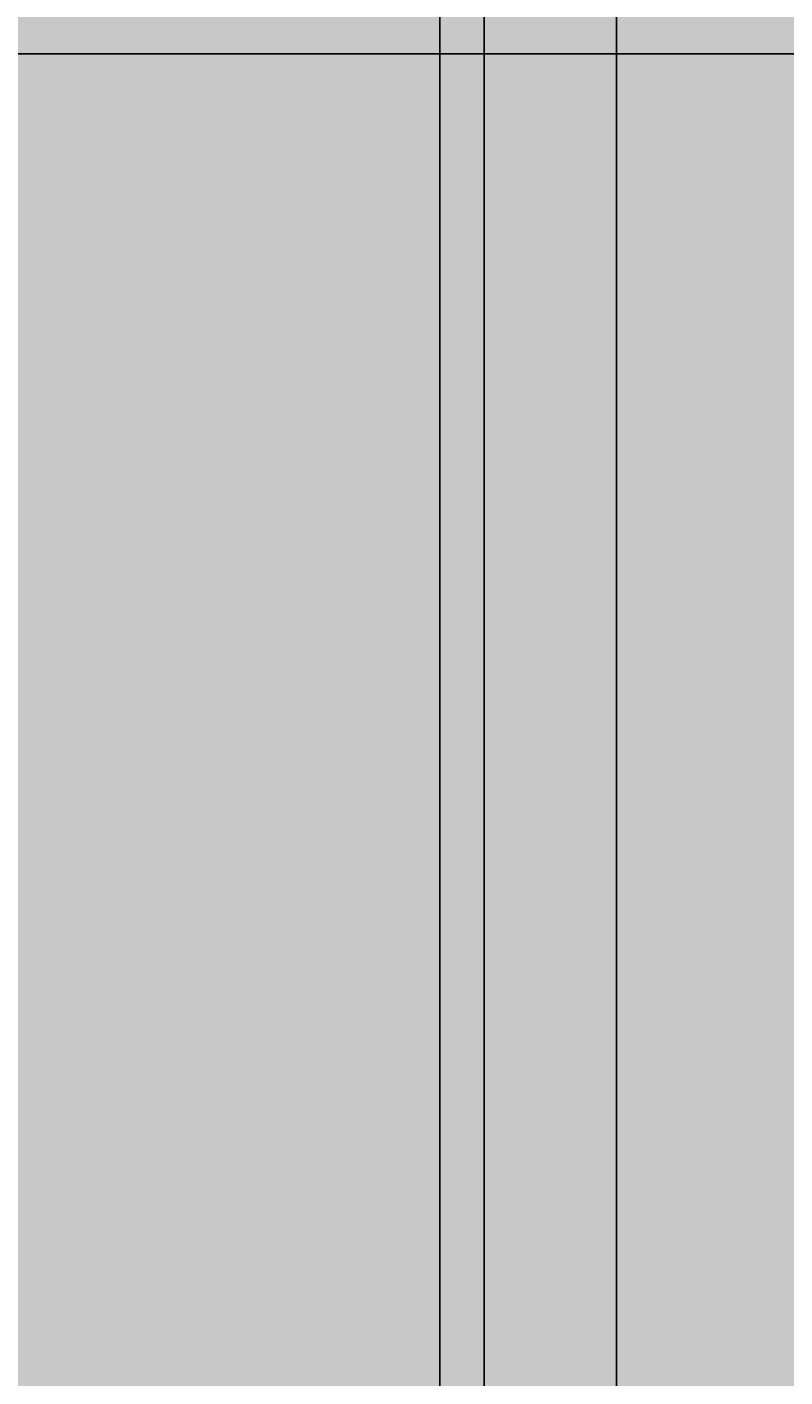
# Model space of a CAD drawing. Units: feet. Extents: x 2695 to 2912, y 795 to 1139.
# Tile 25 of 83: x 2825 to 2842, y 845 to 875. Entities that reach past the tile are written whole.
import ezdxf

# ---------------------------------------------------------------- set-up
doc = ezdxf.new("R2010")
doc.units = ezdxf.units.FT
for name, color, linetype, lineweight in [('A-ANNO-DIMS', 2, 'Continuous', 18), ('A-DOOR', 3, 'Continuous', 25), ('A-DOOR-PATT', 33, 'Continuous', 13), ('A-ELEV-PATT', 252, 'Continuous', 13)]:
    doc.layers.add(name, color=color, linetype=linetype, lineweight=lineweight)
doc.styles.get("Standard").update_dxf_attribs({"font": 'arial.ttf'})
doc.dimstyles.get("Standard").update_dxf_attribs({"dimtxt": 0.18, "dimasz": 0.18, "dimexe": 0.18, "dimexo": 0.0625, "dimgap": 0.09, "dimtad": 0, "dimtih": 1, "dimtoh": 1, "dimdec": 1, "dimzin": 0, "dimdsep": 46, "dimlunit": 3, "dimtxsty": 'Standard', "dimcen": 0.09, "dimadec": 0, "dimazin": 0, "dimtfac": 1, "dimtdec": 1, "dimtofl": 0, "dimtmove": 0, "dimatfit": 3, "dimfxl": 1, "dimtolj": 1, "dimtzin": 0, "dimarcsym": 0})

# ---------------------------------------------------------------- blocks, each defined once
blk = doc.blocks.new('*D13')
at = {"layer": 'A-ANNO-DIMS', "color": 0, "lineweight": -2, "transparency": 16777216}
for p, q in [((2758.214, 874.857), (2911.424, 874.857)), ((2911.244, 874.677), (2911.244, 843.076)), ((2911.244, 811.111), (2911.244, 842.712)), ((2890.699, 810.931), (2911.424, 810.931))]:
    blk.add_line(p, q, dxfattribs=at)
at = {"layer": 'A-ANNO-DIMS', "color": 0, "transparency": 16777216}
for points in [[(2911.214, 874.677), (2911.274, 874.677), (2911.244, 874.857)], [(2911.214, 811.111), (2911.274, 811.111), (2911.244, 810.931)]]:
    blk.add_solid(points, dxfattribs=at)
at = {"layer": 'Defpoints', "color": 0, "transparency": 16777216}
for p in [(2758.151, 874.857), (2911.244, 874.857), (2890.636, 810.931)]:
    blk.add_point(p, dxfattribs=at)
at = {"layer": 'A-ANNO-DIMS', "color": 0, "transparency": 16777216, "insert": (2911.244, 842.894), "char_height": 0.18, "attachment_point": 5}
blk.add_mtext('\\A1;63.93', dxfattribs=at)
blk = doc.blocks.new('*D14')
at = {"layer": 'A-ANNO-DIMS', "color": 0, "lineweight": -2, "transparency": 16777216}
for p, q in [((2838.439, 905.514), (2911.424, 905.514)), ((2911.244, 905.334), (2911.244, 890.368)), ((2911.244, 875.037), (2911.244, 890.004)), ((2758.214, 874.857), (2911.424, 874.857))]:
    blk.add_line(p, q, dxfattribs=at)
at = {"layer": 'A-ANNO-DIMS', "color": 0, "transparency": 16777216}
for points in [[(2911.214, 905.334), (2911.274, 905.334), (2911.244, 905.514)], [(2911.214, 875.037), (2911.274, 875.037), (2911.244, 874.857)]]:
    blk.add_solid(points, dxfattribs=at)
at = {"layer": 'Defpoints', "color": 0, "transparency": 16777216}
for p in [(2838.377, 905.514), (2911.244, 905.514), (2758.151, 874.857)]:
    blk.add_point(p, dxfattribs=at)
at = {"layer": 'A-ANNO-DIMS', "color": 0, "transparency": 16777216, "insert": (2911.244, 890.186), "char_height": 0.18, "attachment_point": 5}
blk.add_mtext('\\A1;30.66', dxfattribs=at)

msp = doc.modelspace()

# ---------------------------------------------------------------- hatches: boundary and pattern name
at = {"layer": 'A-DOOR-PATT'}
h = msp.add_hatch(color=256, dxfattribs=at)
h.set_gradient(color1=(211, 185, 150), color2=(211, 185, 150))
h.paths.add_polyline_path([(2805.9398, 905.5143), (2773.5029, 905.5143), (2773.5029, 810.9306), (2776.4999, 810.9306), (2776.4999, 902.5174), (2802.9429, 902.5174), (2802.9429, 810.9306), (2805.9398, 810.9306)])
h.paths.add_polyline_path([(2803.9681, 874.1057), (2805.0538, 874.1057), (2805.0538, 846.2857), (2803.9681, 846.2857)], flags=16)
h.paths.add_polyline_path([(2838.3767, 905.5143), (2805.9398, 905.5143), (2805.9398, 810.9306), (2808.9368, 810.9306), (2808.9368, 902.5174), (2835.3798, 902.5174), (2835.3798, 810.9306), (2838.3767, 810.9306)])
h = msp.add_hatch(color=256, dxfattribs=at)
h.set_gradient(color1=(211, 185, 150), color2=(211, 185, 150))
h.paths.add_polyline_path([(2777.5029, 901.5143), (2801.9398, 901.5143), (2801.9398, 810.9306), (2802.9429, 810.9306), (2802.9429, 902.5174), (2776.4999, 902.5174), (2776.4999, 810.9306), (2777.5029, 810.9306)])
h.paths.add_polyline_path([(2809.9398, 901.5143), (2834.3767, 901.5143), (2834.3767, 810.9306), (2835.3798, 810.9306), (2835.3798, 902.5174), (2808.9368, 902.5174), (2808.9368, 810.9306), (2809.9398, 810.9306)])
h = msp.add_hatch(color=256, dxfattribs=at)
h.set_gradient(color1=(173, 221, 247), color2=(173, 221, 247))
h.paths.add_polyline_path([(2801.9398, 901.5143), (2777.5029, 901.5143), (2777.5029, 810.9306), (2801.9398, 810.9306)])
h.paths.add_polyline_path([(2834.3767, 901.5143), (2809.9398, 901.5143), (2809.9398, 810.9306), (2834.3767, 810.9306)])
at = {"layer": 'A-ELEV-PATT'}
h = msp.add_hatch(color=256, dxfattribs=at)
h.set_gradient(color1=(147, 149, 152), color2=(147, 149, 152), tint=1)
h.paths.add_polyline_path([(2770.6361, 1118.4096), (2710.6361, 1118.4096), (2710.6361, 1062.9306), (2770.6361, 1062.9306)])
h.paths.add_polyline_path([(2890.6361, 1103.3378), (2770.6361, 1103.3378), (2770.6361, 1062.9306), (2890.6361, 1062.9306)])
h.paths.add_polyline_path([(2730.7081, 1048.1052), (2755.1125, 1048.1052), (2755.1125, 936.9306), (2770.6361, 936.9306), (2770.6361, 1050.3105), (2715.8852, 1050.3105), (2715.8852, 936.9306), (2730.7081, 936.9306)])
h.paths.add_polyline_path([(2890.6361, 1050.3105), (2770.6361, 1050.3105), (2770.6361, 971.9673), (2778.0341, 971.9673), (2778.0341, 1020.8235), (2843.575, 1020.8235), (2843.575, 971.9673), (2890.6361, 971.9673)])
h.paths.add_polyline_path([(2888.1882, 970.7156), (2843.575, 970.7156), (2843.575, 964.8267), (2888.1882, 964.8267)])
h.paths.add_polyline_path([(2888.1882, 964.1328), (2843.575, 964.1328), (2843.575, 956.614), (2888.1882, 956.614)])
h.paths.add_polyline_path([(2888.1882, 955.9202), (2843.575, 955.9202), (2843.575, 949.2892), (2888.1882, 949.2892)])
h.paths.add_polyline_path([(2888.1882, 948.5954), (2843.575, 948.5954), (2843.575, 941.3507), (2888.1882, 941.3507)])
h.paths.add_polyline_path([(2888.1882, 940.6569), (2843.575, 940.6569), (2843.575, 936.9306), (2888.1882, 936.9306)])
h.paths.add_polyline_path([(2890.6361, 970.7156), (2888.9368, 970.7156), (2888.9368, 964.8267), (2890.6361, 964.8267)])
h.paths.add_polyline_path([(2890.6361, 964.1328), (2888.9368, 964.1328), (2888.9368, 956.614), (2890.6361, 956.614)])
h.paths.add_polyline_path([(2890.6361, 955.9202), (2888.9368, 955.9202), (2888.9368, 949.2892), (2890.6361, 949.2892)])
h.paths.add_polyline_path([(2890.6361, 940.6569), (2888.9368, 940.6569), (2888.9368, 936.9306), (2890.6361, 936.9306)])
h.paths.add_polyline_path([(2890.6361, 948.5954), (2888.9368, 948.5954), (2888.9368, 941.3507), (2890.6361, 941.3507)])
h.paths.add_polyline_path([(2772.5216, 970.7156), (2770.6361, 970.7156), (2770.6361, 964.8267), (2772.5216, 964.8267)])
h.paths.add_polyline_path([(2772.5216, 964.1328), (2770.6361, 964.1328), (2770.6361, 956.614), (2772.5216, 956.614)])
h.paths.add_polyline_path([(2772.5216, 955.9202), (2770.6361, 955.9202), (2770.6361, 949.2892), (2772.5216, 949.2892)])
h.paths.add_polyline_path([(2772.5216, 948.5954), (2770.6361, 948.5954), (2770.6361, 941.3507), (2772.5216, 941.3507)])
h.paths.add_polyline_path([(2772.5216, 940.6569), (2770.6361, 940.6569), (2770.6361, 936.9306), (2772.5216, 936.9306)])
h.paths.add_polyline_path([(2778.0341, 940.6569), (2773.2702, 940.6569), (2773.2702, 936.9306), (2778.0341, 936.9306)])
h.paths.add_polyline_path([(2778.0341, 970.7156), (2773.2702, 970.7156), (2773.2702, 964.8267), (2778.0341, 964.8267)])
h.paths.add_polyline_path([(2778.0341, 964.1328), (2773.2702, 964.1328), (2773.2702, 956.614), (2778.0341, 956.614)])
h.paths.add_polyline_path([(2778.0341, 955.9202), (2773.2702, 955.9202), (2773.2702, 949.2892), (2778.0341, 949.2892)])
h.paths.add_polyline_path([(2778.0341, 948.5954), (2773.2702, 948.5954), (2773.2702, 941.3507), (2778.0341, 941.3507)])
h.paths.add_polyline_path([(2810.0407, 940.6569), (2780.0341, 940.6569), (2780.0341, 936.9306), (2810.0407, 936.9306)])
h.paths.add_polyline_path([(2890.6361, 924.3105), (2770.6361, 924.3105), (2770.6361, 810.9306), (2773.5029, 810.9306), (2773.5029, 905.5143), (2805.9398, 905.5143), (2838.3767, 905.5143), (2838.3767, 810.9306), (2890.6361, 810.9306)])

# ---------------------------------------------------------------- linework, layer by layer
at = {"layer": 'A-DOOR'}
for points in [[(2773.5029, 905.5143), (2838.3767, 905.5143), (2838.3767, 810.9306), (2773.5029, 810.9306)], [(2808.9368, 902.5174), (2835.3798, 902.5174), (2835.3798, 810.9306), (2808.9368, 810.9306)], [(2809.9398, 901.5143), (2834.3767, 901.5143), (2834.3767, 810.9306), (2809.9398, 810.9306)]]:
    msp.add_lwpolyline(points, close=True, dxfattribs=at)
for points in [[(2838.3767, 810.9306), (2838.3767, 905.5143), (2805.9398, 905.5143), (2805.9398, 810.9306)], [(2835.3798, 810.9306), (2835.3798, 902.5174), (2808.9368, 902.5174), (2808.9368, 810.9306)], [(2834.3767, 810.9306), (2834.3767, 901.5143), (2809.9398, 901.5143), (2809.9398, 810.9306)]]:
    msp.add_lwpolyline(points, dxfattribs=at)

# ---------------------------------------------------------------- dimensions: what is measured, and where the dimension line sits
at = {"layer": 'A-ANNO-DIMS'}
for base, p1, p2, picture, middle in [((2911.2444, 905.5143), (2758.1515, 874.8571), (2838.3767, 905.5143), '*D14', (2911.2444, 890.1857)), ((2911.2444, 874.8571), (2890.6361, 810.9306), (2758.1515, 874.8571), '*D13', (2911.2444, 842.8938))]:
    dim = msp.add_linear_dim(base=base, p1=p1, p2=p2, angle=90, dimstyle='Standard', override={"dimdec": 2, "dimlfac": 1, "dimrnd": 0, "dimzin": 0, "dimdsep": 46, "dimlunit": 2}, dxfattribs=at)
    dim.commit()
    dim.dimension.update_dxf_attribs({"geometry": picture, "text_midpoint": middle})

doc.saveas('drawing.dxf')
